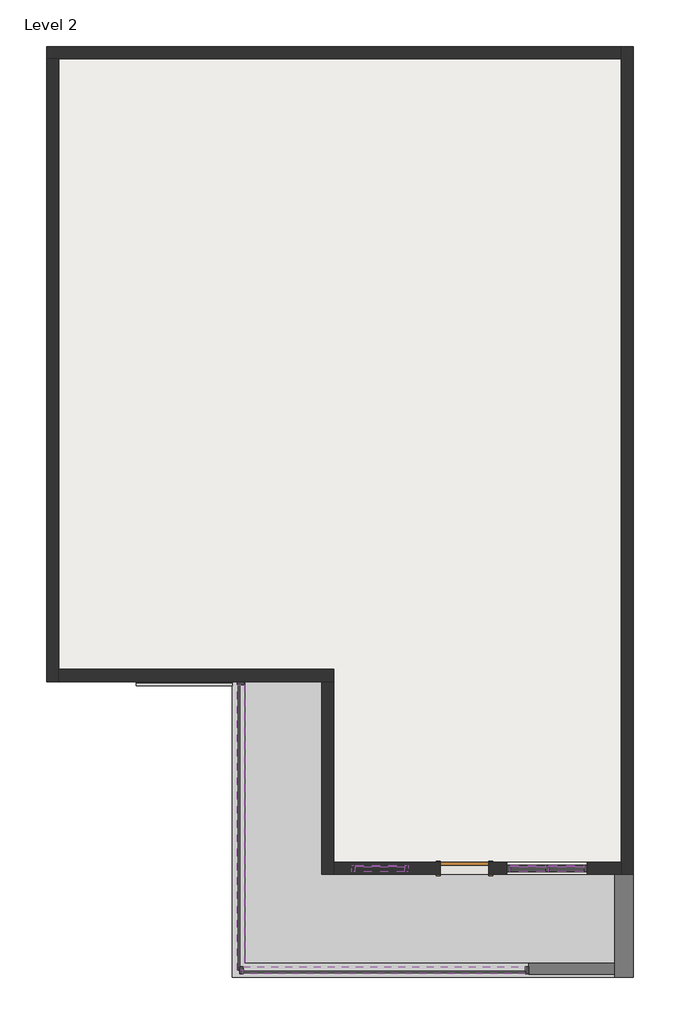
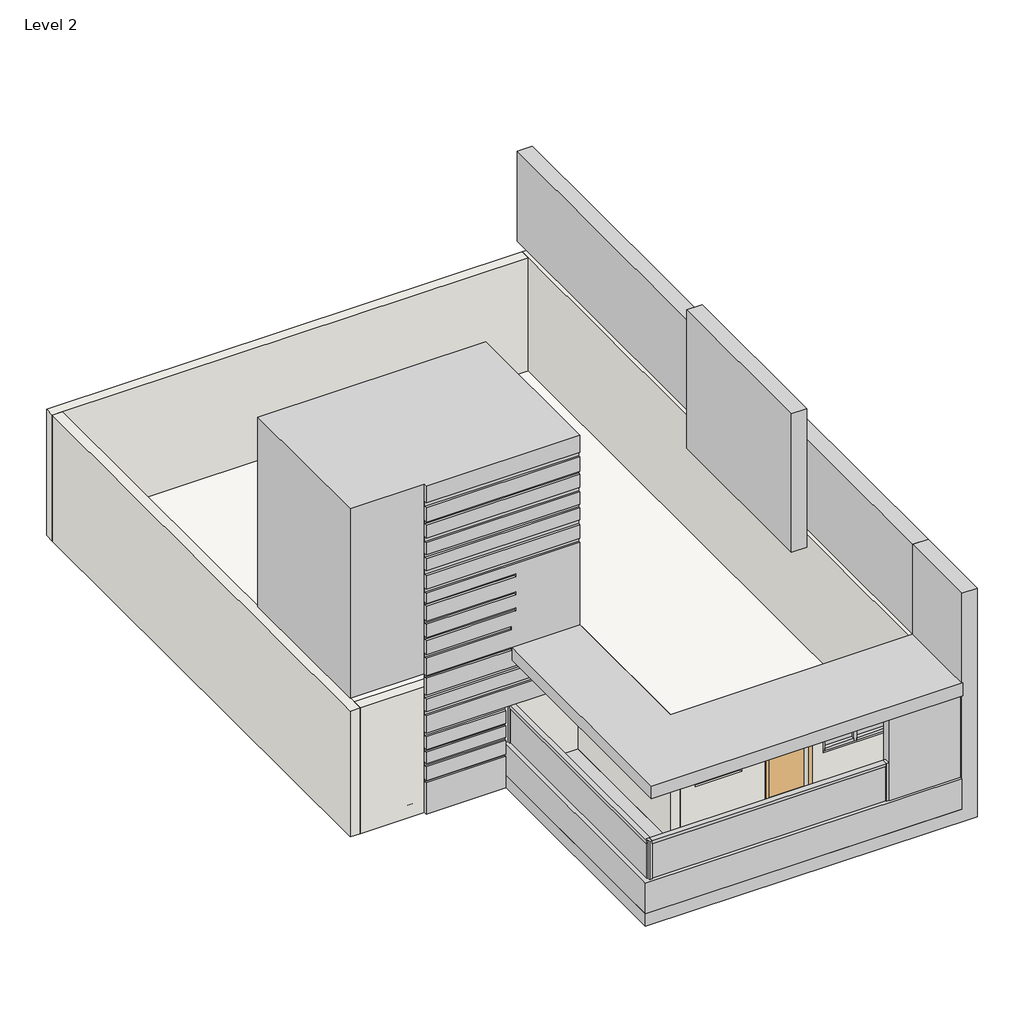
# One storey: 16 members, 6 walls, 5 plates, 2 proxies, 1 door, 1 roof.
"""IFC4 building model written with IfcOpenShell, lengths in millimetres."""

from ifc_helpers import new_model, si_unit, frame, origin, place, context, project, spatial, polyline, outline, extrude, faceted_brep, transform, mapped, element, save
from components import generic_models_2_generic_models_2_8bbb9965, generic_models_7_generic_models_7_2f98df86, door_0ca8825f, member_c33c434a, member_6ba49134, member_48accb65, member_c1b635f4, member_e557a406, member_e78f2157, member_753b68dd, member_614527b7, member_e8a6e381, system_panel_glazed_dcc89d10, system_panel_glazed_0610b94e, system_panel_glazed_b08977a1, system_panel_glazed_aff0b4bd

model = new_model("IFC4")

# Units and contexts
model_context = context("Model", 3, world=origin())
ifc_project = project(units=[si_unit("LENGTHUNIT", "METRE", prefix="MILLI")], contexts=[model_context])

# Site, building, storey
site = spatial("IfcSite", under=ifc_project)
building = spatial("IfcBuilding", under=site)
storey = spatial("IfcBuildingStorey", under=building, Name="Level 2", Elevation=3048.0)

# Proxies
placement = place(None, origin())
generic_models_2_generic_models_2_shape = generic_models_2_generic_models_2_8bbb9965(model_context)
element("IfcBuildingElementProxy", 1, Name="Generic Models 2 : Generic Models 2", ObjectType="Generic Models 2 : Generic Models 2", at=placement, inside=storey, context=model_context, shape_type="MappedRepresentation", body=[
    mapped(generic_models_2_generic_models_2_shape, transform((0.0, 0.0, 0.0), x_axis=(1.0, 0.0, 0.0), y_axis=(0.0, 1.0, 0.0), z_axis=(0.0, 0.0, 1.0))),
])
generic_models_7_generic_models_7_shape = generic_models_7_generic_models_7_2f98df86(model_context)
element("IfcBuildingElementProxy", 2, Name="Generic Models 7 : Generic Models 7", ObjectType="Generic Models 7 : Generic Models 7", at=placement, inside=storey, context=model_context, shape_type="MappedRepresentation", body=[
    mapped(generic_models_7_generic_models_7_shape, transform((0.0, 0.0, 0.0), x_axis=(1.0, 0.0, 0.0), y_axis=(0.0, 1.0, 0.0), z_axis=(0.0, 0.0, 1.0))),
])

# Door
door_shape = door_0ca8825f(model_context)
element("IfcDoor", 3, ObjectType="Single-Flush : 36\" x 84\"", at=placement, inside=storey, context=model_context, shape_type="MappedRepresentation", body=[
    mapped(door_shape, transform((-7952.3321088, -12943.7468404, 3454.4), x_axis=(1.0, 0.0, 0.0), y_axis=(0.0, 1.0, 0.0), z_axis=(0.0, 0.0, 1.0))),
])

# Members
member_shape = member_c33c434a(model_context)
element("IfcMember", 4, ObjectType="Rectangular Mullion : 2.5\" x 5\" rectangular", at=placement, inside=storey, context=model_context, shape_type="MappedRepresentation", body=[
    mapped(member_shape, transform((-6358.4821088, -12943.7468404, 4244.4185547), x_axis=(0.0, 0.0, -1.0), y_axis=(0.0, -1.0, 0.0), z_axis=(-1.0, 0.0, 0.0))),
])
element("IfcMember", 5, ObjectType="Rectangular Mullion : 2.5\" x 5\" rectangular", at=placement, inside=storey, context=model_context, shape_type="MappedRepresentation", body=[
    mapped(member_shape, transform((-7088.7321088, -12943.7468404, 4244.4185547), x_axis=(0.0, 0.0, -1.0), y_axis=(0.0, -1.0, 0.0), z_axis=(-1.0, 0.0, 0.0))),
])
element("IfcMember", 6, ObjectType="Rectangular Mullion : 2.5\" x 5\" rectangular", at=placement, inside=storey, context=model_context, shape_type="MappedRepresentation", body=[
    mapped(member_shape, transform((-6421.9821088, -12943.7468404, 5652.5973882), x_axis=(0.0, 0.0, 1.0), y_axis=(0.0, -1.0, 0.0), z_axis=(1.0, 0.0, 0.0))),
])
element("IfcMember", 7, ObjectType="Rectangular Mullion : 2.5\" x 5\" rectangular", at=placement, inside=storey, context=model_context, shape_type="MappedRepresentation", body=[
    mapped(member_shape, transform((-5691.7321088, -12943.7468404, 5652.5973882), x_axis=(0.0, 0.0, 1.0), y_axis=(0.0, -1.0, 0.0), z_axis=(1.0, 0.0, 0.0))),
])
member_2_shape = member_6ba49134(model_context)
element("IfcMember", 8, ObjectType="Rectangular Mullion : 2.5\" x 5\" rectangular", at=placement, inside=storey, context=model_context, shape_type="MappedRepresentation", body=[
    mapped(member_2_shape, transform((-6390.2321088, -12943.7468404, 4244.4185547), x_axis=(1.0, 0.0, 0.0), y_axis=(0.0, -1.0, 0.0), z_axis=(0.0, 0.0, -1.0))),
])
member_3_shape = member_48accb65(model_context)
element("IfcMember", 9, ObjectType="Rectangular Mullion : 2.5\" x 5\" rectangular", at=placement, inside=storey, context=model_context, shape_type="MappedRepresentation", body=[
    mapped(member_3_shape, transform((-7152.2321088, -12943.7468404, 5652.5973882), x_axis=(-1.0, 0.0, 0.0), y_axis=(0.0, -1.0, 0.0), z_axis=(0.0, 0.0, 1.0))),
])
element("IfcMember", 10, ObjectType="Rectangular Mullion : 2.5\" x 5\" rectangular", at=placement, inside=storey, context=model_context, shape_type="MappedRepresentation", body=[
    mapped(member_3_shape, transform((-5628.2321088, -12943.7468404, 4244.4185547), x_axis=(1.0, 0.0, 0.0), y_axis=(0.0, -1.0, 0.0), z_axis=(0.0, 0.0, -1.0))),
])
member_4_shape = member_c1b635f4(model_context)
element("IfcMember", 11, ObjectType="Rectangular Mullion : 2.5\" x 5\" rectangular", at=placement, inside=storey, context=model_context, shape_type="MappedRepresentation", body=[
    mapped(member_4_shape, transform((-10085.9321088, -12943.7468404, 5596.1256962), x_axis=(-1.0, 0.0, 0.0), y_axis=(0.0, -1.0, 0.0), z_axis=(0.0, 0.0, 1.0))),
])
member_5_shape = member_e557a406(model_context)
element("IfcMember", 12, ObjectType="Rectangular Mullion : 2.5\" x 5\" rectangular", at=placement, inside=storey, context=model_context, shape_type="MappedRepresentation", body=[
    mapped(member_5_shape, transform((-10022.4321088, -12943.7468404, 4453.7765405), x_axis=(0.0, 0.0, -1.0), y_axis=(0.0, -1.0, 0.0), z_axis=(-1.0, 0.0, 0.0))),
])
element("IfcMember", 13, ObjectType="Rectangular Mullion : 2.5\" x 5\" rectangular", at=placement, inside=storey, context=model_context, shape_type="MappedRepresentation", body=[
    mapped(member_5_shape, transform((-9082.6321088, -12943.7468404, 5596.1256962), x_axis=(0.0, 0.0, 1.0), y_axis=(0.0, -1.0, 0.0), z_axis=(1.0, 0.0, 0.0))),
])
element("IfcMember", 14, ObjectType="Rectangular Mullion : 2.5\" x 5\" rectangular", at=placement, inside=storey, context=model_context, shape_type="MappedRepresentation", body=[
    mapped(member_4_shape, transform((-9019.1321088, -12943.7468404, 4453.7765405), x_axis=(1.0, 0.0, 0.0), y_axis=(0.0, -1.0, 0.0), z_axis=(0.0, 0.0, -1.0))),
])
member_6_shape = member_e78f2157(model_context)
element("IfcMember", 15, ObjectType="Rectangular Mullion : 2.5\" x 5\" rectangular", at=placement, inside=storey, context=model_context, shape_type="MappedRepresentation", body=[
    mapped(member_6_shape, transform((-12215.152412, -14875.2784039, 3733.8751937), x_axis=(-1.0, 0.0, 0.0), y_axis=(0.0, 1.0, 0.0), z_axis=(0.0, 0.0, -1.0))),
])
member_7_shape = member_753b68dd(model_context)
element("IfcMember", 16, ObjectType="Rectangular Mullion : 2.5\" x 5\" rectangular", at=placement, inside=storey, context=model_context, shape_type="MappedRepresentation", body=[
    mapped(member_7_shape, transform((-12196.102412, -9463.9468404, 5004.8316632), x_axis=(0.0, 0.0, 1.0), y_axis=(1.0, 0.0, 0.0), z_axis=(0.0, 1.0, 0.0))),
])
member_8_shape = member_614527b7(model_context)
element("IfcMember", 17, ObjectType="Rectangular Mullion : 2.5\" x 5\" rectangular", at=placement, inside=storey, context=model_context, shape_type="MappedRepresentation", body=[
    mapped(member_8_shape, transform((-12196.102412, -9400.4468404, 3585.7685561), x_axis=(0.0, 1.0, 0.0), y_axis=(1.0, 0.0, 0.0), z_axis=(0.0, 0.0, -1.0))),
])
member_9_shape = member_e8a6e381(model_context)
element("IfcMember", 18, ObjectType="Rectangular Mullion : 2.5\" x 5\" rectangular", at=placement, inside=storey, context=model_context, shape_type="MappedRepresentation", body=[
    mapped(member_9_shape, transform((-12151.652412, -14875.2784039, 5004.8316632), x_axis=(0.0, 0.0, 1.0), y_axis=(0.0, 1.0, 0.0), z_axis=(-1.0, 0.0, 0.0))),
])
element("IfcMember", 19, ObjectType="Rectangular Mullion : 2.5\" x 5\" rectangular", at=placement, inside=storey, context=model_context, shape_type="MappedRepresentation", body=[
    mapped(member_6_shape, transform((-6735.102412, -14875.2784039, 5004.8316632), x_axis=(1.0, 0.0, 0.0), y_axis=(0.0, 1.0, 0.0), z_axis=(0.0, 0.0, 1.0))),
])

# Plates
system_panel_glazed_shape = system_panel_glazed_dcc89d10(model_context)
element("IfcPlate", 20, ObjectType="System Panel : Glazed", at=placement, inside=storey, context=model_context, shape_type="MappedRepresentation", body=[
    mapped(system_panel_glazed_shape, transform((-6755.3571088, -12943.7468404, 4307.9185547), x_axis=(1.0, 0.0, 0.0), y_axis=(0.0, 1.0, 0.0), z_axis=(0.0, 0.0, 1.0))),
])
element("IfcPlate", 21, ObjectType="System Panel : Glazed", at=placement, inside=storey, context=model_context, shape_type="MappedRepresentation", body=[
    mapped(system_panel_glazed_shape, transform((-6025.1071088, -12943.7468404, 4307.9185547), x_axis=(1.0, 0.0, 0.0), y_axis=(0.0, 1.0, 0.0), z_axis=(0.0, 0.0, 1.0))),
])
system_panel_glazed_2_shape = system_panel_glazed_0610b94e(model_context)
element("IfcPlate", 22, ObjectType="System Panel : Glazed", at=placement, inside=storey, context=model_context, shape_type="MappedRepresentation", body=[
    mapped(system_panel_glazed_2_shape, transform((-9552.5321088, -12943.7468404, 4517.2765405), x_axis=(1.0, 0.0, 0.0), y_axis=(0.0, 1.0, 0.0), z_axis=(0.0, 0.0, 1.0))),
])
system_panel_glazed_3_shape = system_panel_glazed_b08977a1(model_context)
element("IfcPlate", 23, ObjectType="System Panel : Glazed", at=placement, inside=storey, context=model_context, shape_type="MappedRepresentation", body=[
    mapped(system_panel_glazed_3_shape, transform((-12196.102412, -12169.6126222, 3585.7685561), x_axis=(0.0, 1.0, 0.0), y_axis=(-1.0, 0.0, 0.0), z_axis=(0.0, 0.0, 1.0))),
])
system_panel_glazed_4_shape = system_panel_glazed_aff0b4bd(model_context)
element("IfcPlate", 24, ObjectType="System Panel : Glazed", at=placement, inside=storey, context=model_context, shape_type="MappedRepresentation", body=[
    mapped(system_panel_glazed_4_shape, transform((-9475.127412, -14875.2784039, 3733.8751937), x_axis=(-1.0, 0.0, 0.0), y_axis=(0.0, -1.0, 0.0), z_axis=(0.0, 0.0, 1.0))),
])

# Roof
element("IfcRoof", 25, ObjectType="Generic - 12\"", at=placement, inside=storey, context=model_context, shape_type="SweptSolid", body=[
    extrude(outline(polyline([(-15877.1321088, 2639.1531596), (-4751.9321088, 2639.1531596), (-4751.9321088, -13058.0468404), (-10657.4321088, -13058.0468404), (-10657.4321088, -9400.4468404), (-15877.1321088, -9400.4468404), (-15877.1321088, 2639.1531596)])), frame((0.0, 0.0, 3048.0), z_axis=(0.0, 0.0, 1.0), x_axis=(1.0, 0.0, 0.0)), (0.0, 0.0, 1.0), 304.8),
])

# Walls
element("IfcWall", 26, ObjectType="9\"", at=placement, inside=storey, context=model_context, shape_type="Brep", body=[
    faceted_brep([(-4751.9321088, -13058.0468404, 3048.0), (-4751.9321088, 2639.1531596, 3048.0), (-4751.9321088, 2639.1531596, 6096.0), (-4751.9321088, -13058.0468404, 6096.0), (-4980.5321088, -13058.0468404, 3048.0), (-4980.5321088, -13058.0468404, 6096.0), (-4980.5321088, -12829.4468404, 6096.0), (-4980.5321088, 2410.5531596, 6096.0), (-4980.5321088, 2639.1531596, 6096.0), (-4980.5321088, 2639.1531596, 3048.0), (-4980.5321088, 2410.5531596, 3048.0), (-4980.5321088, -12829.4468404, 3048.0)], [[[0, 1, 2, 3]], [[4, 5, 6, 7, 8, 9, 10, 11]], [[1, 0, 4, 11, 10, 9]], [[3, 2, 8, 7, 6, 5]], [[2, 1, 9, 8]], [[0, 3, 5, 4]]]),
])
element("IfcWall", 27, ObjectType="9\"", at=placement, inside=storey, context=model_context, shape_type="Brep", body=[
    faceted_brep([(-4980.5321088, 2639.1531596, 3048.0), (-15877.1321088, 2639.1531596, 3048.0), (-15877.1321088, 2639.1531596, 6096.0), (-4980.5321088, 2639.1531596, 6096.0), (-4980.5321088, 2410.5531596, 3048.0), (-4980.5321088, 2410.5531596, 6096.0), (-15648.5321088, 2410.5531596, 6096.0), (-15877.1321088, 2410.5531596, 6096.0), (-15877.1321088, 2410.5531596, 3048.0), (-15648.5321088, 2410.5531596, 3048.0)], [[[0, 1, 2, 3]], [[4, 5, 6, 7, 8, 9]], [[1, 0, 4, 9, 8]], [[3, 2, 7, 6, 5]], [[0, 3, 5, 4]], [[2, 1, 8, 7]]]),
])
element("IfcWall", 28, ObjectType="9\"", at=placement, inside=storey, context=model_context, shape_type="Brep", body=[
    faceted_brep([(-15877.1321088, 2410.5531596, 3048.0), (-15877.1321088, -9400.4468404, 3048.0), (-15877.1321088, -9400.4468404, 6096.0), (-15877.1321088, 2410.5531596, 6096.0), (-15648.5321088, 2410.5531596, 3048.0), (-15648.5321088, 2410.5531596, 6096.0), (-15648.5321088, -9171.8468404, 6096.0), (-15648.5321088, -9400.4468404, 6096.0), (-15648.5321088, -9400.4468404, 3048.0), (-15648.5321088, -9171.8468404, 3048.0)], [[[0, 1, 2, 3]], [[4, 5, 6, 7, 8, 9]], [[1, 0, 4, 9, 8]], [[3, 2, 7, 6, 5]], [[0, 3, 5, 4]], [[2, 1, 8, 7]]]),
])
element("IfcWall", 29, ObjectType="9\"", at=placement, inside=storey, context=model_context, shape_type="Brep", body=[
    faceted_brep([(-15648.5321088, -9400.4468404, 3048.0), (-10657.4321088, -9400.4468404, 3048.0), (-10428.8321088, -9400.4468404, 3048.0), (-10428.8321088, -9400.4468404, 6096.0), (-10657.4321088, -9400.4468404, 6096.0), (-15648.5321088, -9400.4468404, 6096.0), (-15648.5321088, -9171.8468404, 3048.0), (-15648.5321088, -9171.8468404, 6096.0), (-10428.8321088, -9171.8468404, 6096.0), (-10428.8321088, -9171.8468404, 3048.0)], [[[0, 1, 2, 3, 4, 5]], [[6, 7, 8, 9]], [[2, 1, 0, 6, 9]], [[5, 4, 3, 8, 7]], [[0, 5, 7, 6]], [[3, 2, 9, 8]]]),
])
element("IfcWall", 30, ObjectType="9\"", at=placement, inside=storey, context=model_context, shape_type="Brep", body=[
    faceted_brep([(-10657.4321088, -9400.4468404, 3048.0), (-10657.4321088, -13058.0468404, 3048.0), (-10657.4321088, -13058.0468404, 6096.0), (-10657.4321088, -9400.4468404, 6096.0), (-10428.8321088, -9400.4468404, 3048.0), (-10428.8321088, -9400.4468404, 6096.0), (-10428.8321088, -12829.4468404, 6096.0), (-10428.8321088, -13058.0468404, 6096.0), (-10428.8321088, -13058.0468404, 3048.0), (-10428.8321088, -12829.4468404, 3048.0)], [[[0, 1, 2, 3]], [[4, 5, 6, 7, 8, 9]], [[1, 0, 4, 9, 8]], [[3, 2, 7, 6, 5]], [[0, 3, 5, 4]], [[2, 1, 8, 7]]]),
])
element("IfcWall", 31, ObjectType="9\"", at=placement, inside=storey, context=model_context, shape_type="SweptSolid", body=[
    extrude(outline(polyline([(3048.0, -10428.8321088), (3048.0, -4980.5321088), (6096.0, -4980.5321088), (6096.0, -10428.8321088), (3048.0, -10428.8321088)]), holes=[polyline([(4453.7765405, -10085.9321088), (5596.1256962, -10085.9321088), (5596.1256962, -9019.1321088), (4453.7765405, -9019.1321088), (4453.7765405, -10085.9321088)]), polyline([(3454.4, -7495.1321088), (3454.4, -8409.5321088), (5588.0, -8409.5321088), (5588.0, -7495.1321088), (3454.4, -7495.1321088)]), polyline([(4244.4185547, -7152.2321088), (5652.5973882, -7152.2321088), (5652.5973882, -5628.2321088), (4244.4185547, -5628.2321088), (4244.4185547, -7152.2321088)])]), frame((0.0, -13058.0468404, 0.0), z_axis=(0.0, 1.0, 0.0), x_axis=(0.0, 0.0, 1.0)), (0.0, 0.0, 1.0), 228.6),
])

save(model, "model.ifc")

# Revit data of these elements
# Type "Single-Flush : 36\" x 84\""
#   Type Mark = "1"
#   Construction Type Id = "MDOOR"
#   Assembly Code = "C1020"
#   Analytic Construction = "Metal"
#   Thickness = 0' - 2"
#   Heat Transfer Coefficient (U) = 0.651978 BTU/(h·ft²·°F)
#   Height = 7' - 0"
#   Trim Projection Ext = 0' - 1"
#   Trim Projection Int = 0' - 1"
#   Trim Width = 0' - 3"
#   Width = 3' - 0"
#   Define Thermal Properties by = 1
#   Define Thermal Properties by = 1
#   Door Material = Door - Panel
#   Frame Material = Door - Frame
#   Visual Light Transmittance = 0
#   Solar Heat Gain Coefficient = 0
#   Function = (empty or 0)
#   Wall Closure = (empty or 0)
# Type "Rectangular Mullion : 2.5\" x 5\" rectangular"
#   built-in parameter 1007304 = 0.416667 (stored number, unit not read)
#   built-in parameter 1007301 = 0.104167 (stored number, unit not read)
#   built-in parameter 1007300 = 0.104167 (stored number, unit not read)
# Type "System Panel : Glazed"
#   Construction Type Id = "GSP4R"
#   Analytic Construction = "1/8 in Pilkington single glazing"
#   Visual Light Transmittance = 0.9
#   Solar Heat Gain Coefficient = 0.86
#   Heat Transfer Coefficient (U) = 1.18115 BTU/(h·ft²·°F)
#   Define Thermal Properties by = 1
# Type "Generic - 12\""
#   Assembly Code = "B1020"
#   Layers, outside or top first: 1' - 0" no material (function 1)
# Type "9\""
#   Assembly Code = "B2010"
#   Layers, outside or top first: 0' - 9" no material (function 1)
# Element 1 (IfcBuildingElementProxy, "Generic Models 2 : Generic Models 2")
#   Phase Created = New Construction
# Element 2 (IfcBuildingElementProxy, "Generic Models 7 : Generic Models 7")
#   Phase Created = New Construction
# Element 3 (IfcDoor, "Single-Flush : 36\" x 84\"")
#   Phase Created = New Construction
#   Materials on its faces: "Door - Frame", "Door - Panel"
# Elements 4, 5, 6, 7, 8, 9, 10, 11, 12, 13, 14, 15, 16, 17, 18, 19 (IfcMember, "Rectangular Mullion : 2.5\" x 5\" rectangular")
#   Phase Created = New Construction
#   Materials on its faces: "Aluminum"
# Elements 20, 21, 22, 23, 24 (IfcPlate, "System Panel : Glazed")
#   Phase Created = New Construction
#   Materials on its faces: "Glass"
# Element 25 (IfcRoof, "Generic - 12\"")
#   built-in parameter 1001705 = 11 (stored number, unit not read)
#   built-in parameter 1001710 = 33615
#   Phase Created = New Construction
#   Materials on its faces: "Default Roof"
# Elements 26, 27, 28, 29, 30, 31 (IfcWall, "9\"")
#   Top Offset = 0' - 0"
#   Base Offset = 0' - 0"
#   Unconnected Height = 10' - 0"
#   wall height = 10' - 0"
#   Phase Created = New Construction
#   Base Constraint = Level 2
#   Materials on its faces: "Default Wall"
# Materials
#   "Door - Panel": class "Wood", colour RGB 210 159 95, transparency 0, Cost = 0
#   "Door - Frame": colour RGB 118 70 51, transparency 0, Cost = 0
#   "Aluminum": class "Metal", colour RGB 247 247 247, transparency 0, Description = "Aluminum 6061", Cost = 0
#   "Glass": class "Glass", colour RGB 0 128 192, transparency 0.75, Description = "Soda Lime Glass", Cost = 0
#   "Default Roof": colour RGB 88 101 114, transparency 0, Cost = 0
#   "Default Wall": colour RGB 128 128 128, transparency 0, Cost = 0
